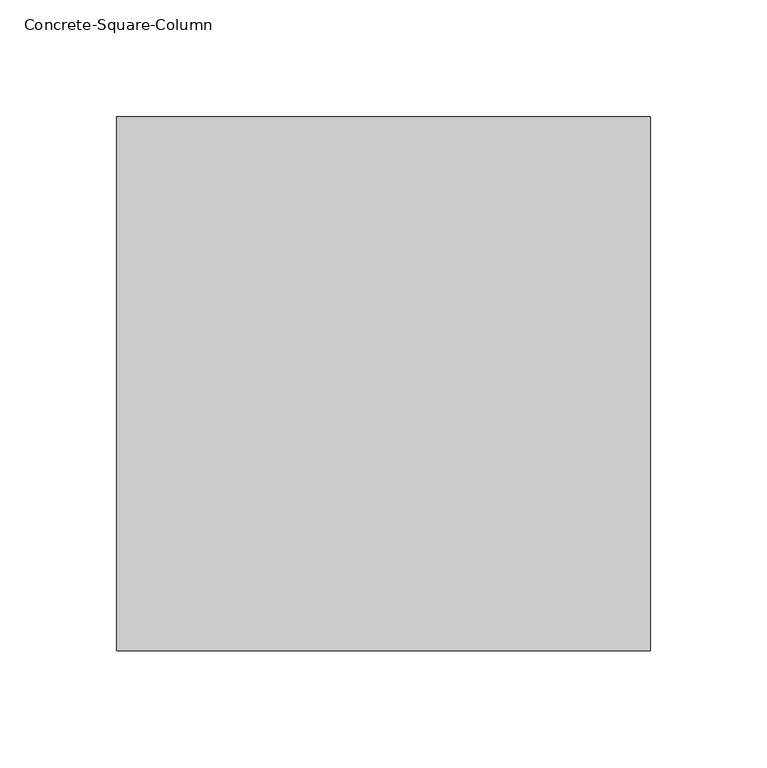
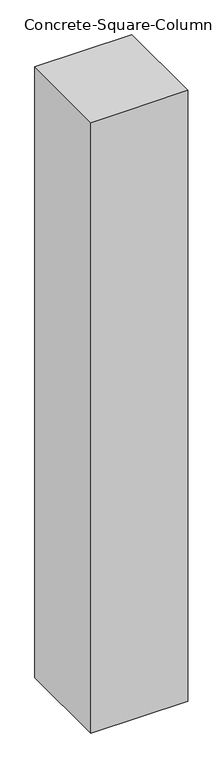
"""IFC4 building model written with IfcOpenShell, lengths in millimetres: column geometry, Concrete-Square-Column."""

from ifc_helpers import new_model, si_unit, frame, origin, place, context, project, spatial, polyline, outline, extrude, source, transform, mapped, element, save


def concrete_square_column_fdf53bfc(model_context):
    return source(origin(), model_context, "Body", "SweptSolid", [
        extrude(outline(polyline([(114.3, 114.3), (114.3, -114.3), (-114.3, -114.3), (-114.3, 114.3), (114.3, 114.3)])), frame((0.0, 0.0, 609.6), z_axis=(0.0, 0.0, 1.0), x_axis=(1.0, 0.0, 0.0)), (0.0, 0.0, 1.0), 1524.0),
    ])


if __name__ == "__main__":
    model = new_model("IFC4")
    model_context = context("Model", 3, world=origin())
    ifc_project = project(units=[si_unit("LENGTHUNIT", "METRE", prefix="MILLI")], contexts=[model_context])
    site = spatial("IfcSite", under=ifc_project)
    building = spatial("IfcBuilding", under=site)
    placement = place(None, origin())
    concrete_square_column_shape = concrete_square_column_fdf53bfc(model_context)
    element("IfcColumn", 1, ObjectType="Concrete-Square-Column", at=placement, inside=building, context=model_context, shape_type="MappedRepresentation", body=[
        mapped(concrete_square_column_shape, transform((0.0, 0.0, 0.0), x_axis=(1.0, 0.0, 0.0), y_axis=(0.0, 1.0, 0.0), z_axis=(0.0, 0.0, 1.0))),
    ])
    save(model, "model.ifc")

# Revit data of these elements
# Type "Concrete-Square-Column"
#   Assembly Code = "B10"
#   b = 0' - 9"
#   Structural Material [instance default] = Concrete, Cast-in-Place gray
# Element 1 (IfcColumn, "Concrete-Square-Column")
#   Materials on its faces: "Concrete, Cast-in-Place gray"
# Materials
#   "Concrete, Cast-in-Place gray": class "Concrete", colour RGB 192 192 192, transparency 0, Description = "Cast-in-place concrete", Cost = 0
